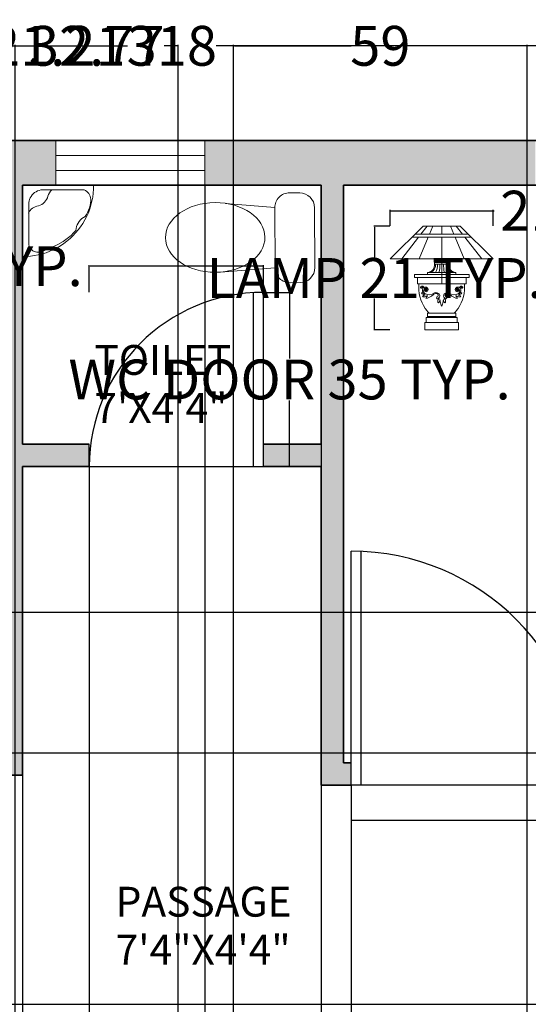
# Model space of a CAD drawing. Units: inches. Extents: x -24 to 368, y -370 to 58.
# Tile 8 of 9: x 133 to 235, y -140 to 58. Entities that reach past the tile are written whole.
import ezdxf

# ---------------------------------------------------------------- set-up
doc = ezdxf.new("R2010")
doc.units = ezdxf.units.IN
doc.header["$MEASUREMENT"] = 0
for name, color, linetype, lineweight in [('A-ANNO-DIMS', 2, 'Continuous', 18), ('A-AREA-IDEN', 7, 'Continuous', 18), ('A-FLOR-FIXT', 8, 'Continuous', 18), ('A-WALL', 7, 'Continuous', 35), ('Furniture', 7, 'Continuous', 15)]:
    doc.layers.add(name, color=color, linetype=linetype, lineweight=lineweight)
for name, color, linetype, lineweight, true_color in [('A-DOOR', 40, 'Continuous', 25, 0xf8d731), ('A-GLAZ', 30, 'Continuous', 18, 0xf26722), ('A-WALL-PATT', 18, 'Continuous', 13, 0x000000)]:
    doc.layers.add(name, color=color, linetype=linetype, lineweight=lineweight, true_color=true_color)
doc.styles.get("Standard").update_dxf_attribs({"font": 'arial.ttf'})
doc.dimstyles.get("Standard").update_dxf_attribs({"dimtxt": 8, "dimasz": 0.18, "dimexe": 0.18, "dimexo": 0.0625, "dimgap": 0.09, "dimtad": 0, "dimtih": 1, "dimtoh": 1, "dimdec": 4, "dimzin": 0, "dimdsep": 46, "dimlunit": 3, "dimtxsty": 'Standard', "dimcen": 0.09, "dimclre": 5, "dimclrt": 6, "dimadec": 0, "dimazin": 0, "dimtfac": 1, "dimtdec": 4, "dimtofl": 0, "dimtmove": 0, "dimatfit": 3, "dimfxl": 1, "dimtolj": 1, "dimtzin": 0, "dimarcsym": 0})

# ---------------------------------------------------------------- blocks, each defined once
blk = doc.blocks.new('LAMP-BEDSIDE')
for p, q in [((6.65, 20.8), (0, 14.26)), ((6.17, 19.19), (7.42, 20.8)), ((6.65, 20.8), (14.09, 20.8)), ((8.59, 20.8), (7.91, 19.19)), ((10.37, 20.8), (10.37, 19.19)), ((12.15, 20.8), (12.83, 19.19)), ((14.57, 19.19), (13.31, 20.8)), ((14.09, 20.8), (20.74, 14.26)), ((2.33, 14.26), (5.71, 18.6)), ((4.42, 18.6), (16.32, 18.6)), ((5.01, 19.19), (15.72, 19.19)), ((7.66, 18.6), (5.82, 14.26)), ((10.37, 18.6), (10.37, 9.21)), ((13.08, 18.6), (14.92, 14.26)), ((18.41, 14.26), (15.02, 18.6)), ((0, 14.26), (20.74, 14.26)), ((9.6, 14.09), (11.14, 14.09)), ((9.6, 14.09), (9.6, 13.52)), ((11.14, 14.09), (11.14, 13.52)), ((8.92, 13.52), (11.81, 13.52)), ((8.92, 13.52), (8.92, 13.19)), ((8.92, 13.19), (11.81, 13.19)), ((11.81, 13.52), (11.81, 13.19)), ((4.88, 11.13), (4.88, 10.49)), ((4.88, 11.13), (15.86, 11.13)), ((4.88, 10.49), (15.86, 10.49)), ((5.48, 10.49), (5.48, 9.21)), ((7.53, 11.52), (13.2, 11.52)), ((7.53, 11.52), (7.53, 11.13)), ((13.2, 11.52), (13.2, 11.13)), ((15.26, 10.49), (15.26, 9.21)), ((15.86, 11.13), (15.86, 10.49)), ((5.48, 9.21), (15.26, 9.21)), ((5.76, 9.21), (5.76, 8.59)), ((14.98, 9.21), (14.98, 8.59)), ((7.24, 2.43), (10.37, 2.43)), ((7.24, 2.43), (7.24, 1.48)), ((7.53, 3.34), (10.37, 3.34)), ((7.53, 3.34), (7.53, 2.65)), ((7.53, 2.65), (10.37, 2.65)), ((13.2, 3.34), (10.37, 3.34)), ((13.2, 2.65), (10.37, 2.65)), ((13.5, 2.43), (10.37, 2.43)), ((13.2, 3.34), (13.2, 2.65)), ((13.5, 2.43), (13.5, 1.48)), ((6.96, 1.48), (6.96, 0)), ((6.96, 1.48), (7.24, 1.48)), ((6.96, 0), (10.37, 0)), ((7.24, 1.48), (10.37, 1.48)), ((13.5, 1.48), (10.37, 1.48)), ((13.77, 0), (10.37, 0)), ((13.77, 1.48), (13.5, 1.48)), ((13.77, 1.48), (13.77, 0))]:
    blk.add_line(p, q)
for centre, radius, start, end in [((7.4, 13.04), 1.53, 274.9221, 5.4044), ((7.51, 13), 1.63, 295.0919, 6.6681), ((6.74, 12.97), 2.77, 328.5732, 4.5839), ((4.28, 12.92), 5.72, 345.8511, 2.7031), ((16.46, 12.92), 5.72, 177.2969, 194.1489), ((14, 12.97), 2.77, 175.4161, 211.4268), ((13.22, 13), 1.63, 173.3319, 244.9081), ((13.33, 13.04), 1.53, 174.5956, 265.0779), ((13.2, 8.5), 7.44, 179.3119, 219.4824), ((6.29, 8.51), 0.158, 124.9924, 335.335), ((6.45, 8.39), 0.355, 11.1092, 135.0155), ((6.39, 8.42), 0.0502, 145.048, 23.2806), ((6.51, 8.39), 0.171, 352.7452, 159.4145), ((7.39, 7.88), 0.87, 145.6908, 234.6789), ((7.4, 7.83), 0.668, 137.9008, 234.3868), ((7.12, 8.07), 0.5, 320.8911, 130.3323), ((7.11, 7.94), 0.236, 29.1955, 234.854), ((7.14, 8.08), 0.309, 326.7711, 139.3622), ((7.2, 8), 0.128, 26.7504, 223.4128), ((13.61, 8.07), 0.5, 49.6677, 219.1089), ((7.54, 8.5), 7.44, 320.5176, 0.6881), ((13.6, 8.08), 0.309, 40.6378, 213.2289), ((13.63, 7.94), 0.236, 305.146, 150.8045), ((13.54, 8), 0.128, 316.5872, 153.2496), ((13.34, 7.83), 0.668, 305.6132, 42.0992), ((13.34, 7.88), 0.87, 305.3211, 34.3092), ((14.29, 8.39), 0.355, 44.9845, 168.8908), ((14.23, 8.39), 0.171, 20.5855, 187.2548), ((14.45, 8.51), 0.158, 204.665, 55.0076), ((14.35, 8.42), 0.0502, 156.7194, 34.952), ((6.44, 6.9), 0.527, 30.7639, 106.5031), ((6.66, 7.53), 0.391, 199.4301, 258.0626), ((6.99, 6.45), 0.534, 81.7725, 150.3347), ((6.86, 7.15), 0.552, 231.7834, 300.6647), ((6.55, 6.3), 0.85, 53.0509, 88.4488), ((7.24, 8), 0.363, 223.4201, 318.9658), ((7.88, 8.48), 1.48, 232.7522, 313.7075), ((7.25, 8.05), 0.203, 224.103, 315.897), ((7.49, 6.32), 0.495, 75.8737, 133.8842), ((7.68, 6.3), 0.502, 98.3136, 177.606), ((7.04, 8.37), 2.05, 274.0547, 309.0162), ((5.53, 10.82), 4.92, 304.6293, 311.2979), ((9.22, 6.66), 0.644, 58.6818, 132.9572), ((9.12, 6.87), 0.587, 71.5671, 111.734), ((9.36, 6.81), 0.621, 342.0461, 94.8157), ((9.69, 6.38), 0.339, 108.5318, 204.8769), ((9.33, 6.92), 0.689, 273.9841, 333.6418), ((9.32, 6.94), 0.352, 316.7375, 49.0095), ((10.14, 5.79), 0.564, 138.2432, 224.6957), ((9.31, 6.66), 0.643, 310.3655, 356.3809), ((8.93, 6.11), 1.09, 318.697, 356.3018), ((9.3, 5.7), 0.788, 353.0671, 25.9825), ((11.43, 5.7), 0.788, 154.0175, 186.9329), ((11.81, 6.11), 1.09, 183.6982, 221.303), ((11.38, 6.81), 0.621, 85.1843, 197.9539), ((11.41, 6.92), 0.689, 206.3582, 266.0159), ((11.43, 6.66), 0.643, 183.6191, 229.6345), ((10.59, 5.79), 0.564, 315.3043, 41.7568), ((11.41, 6.94), 0.352, 130.9905, 223.2625), ((11.05, 6.38), 0.339, 335.1231, 71.4682), ((11.52, 6.66), 0.644, 47.0428, 121.3182), ((11.62, 6.87), 0.587, 68.266, 108.4329), ((12.85, 8.48), 1.48, 226.2925, 307.2478), ((15.2, 10.82), 4.92, 228.7021, 235.3707), ((13.7, 8.37), 2.05, 230.9838, 265.9453), ((13.25, 6.32), 0.495, 46.1158, 104.1263), ((13.05, 6.3), 0.502, 2.394, 81.6864), ((13.5, 8), 0.363, 221.0342, 316.5799), ((13.48, 8.05), 0.203, 224.103, 315.897), ((13.87, 7.15), 0.552, 239.3353, 308.2166), ((14.18, 6.3), 0.85, 91.5512, 126.9491), ((13.75, 6.45), 0.534, 29.6653, 98.2275), ((14.3, 6.9), 0.527, 73.4969, 149.2361), ((14.08, 7.53), 0.391, 281.9374, 340.5699), ((12.16, 5.83), 2.09, 186.3334, 210.8958), ((8.58, 5.83), 2.09, 329.1042, 353.6666), ((7.29, 2.67), 0.245, 257.4164, 350.592), ((10.43, 6.05), 3.74, 217.4462, 226.2556), ((10.31, 6.05), 3.74, 313.7444, 322.5538), ((10.31, 6.05), 3.74, 313.7444, 322.5538), ((13.45, 2.67), 0.245, 189.408, 282.5836)]:
    blk.add_arc(centre, radius, start, end)
blk = doc.blocks.new('WINDOW-30')
for p, q in [((0, 9), (30, 9)), ((0, 0), (0, 9)), ((30, 9), (30, 0)), ((0, 6), (30, 6)), ((0, 3), (30, 3)), ((30, 0), (0, 0))]:
    blk.add_line(p, q)
blk = doc.blocks.new('DOOR-SINGLE-35')
for p, q in [((0, 35), (0, 0)), ((0, 35), (4.5, 35)), ((0, 2), (35, 2)), ((0, 0), (35, 0)), ((0, 0), (4.5, 0))]:
    blk.add_line(p, q)
blk.add_arc((0, 0), 35, 0, 90)
blk = doc.blocks.new('DOOR-SINGLE-47')
for p, q in [((0, 0), (0, 47)), ((2, 0), (2, 47)), ((47, 0), (0, 0))]:
    blk.add_line(p, q)
blk.add_arc((0, 0), 47, 0, 90)
blk = doc.blocks.new('*D13')
at = {"layer": 'A-ANNO-DIMS', "color": 5, "lineweight": -2, "transparency": 16777216}
for p, q in [((206.97, 16.43), (203.73, 16.43)), ((206.97, -4.37), (203.73, -4.37))]:
    blk.add_line(p, q, dxfattribs=at)
at = {"layer": 'A-ANNO-DIMS', "color": 0, "lineweight": -2, "transparency": 16777216}
for p, q in [((203.91, 16.25), (203.91, 10.14)), ((203.91, -4.19), (203.91, 1.92))]:
    blk.add_line(p, q, dxfattribs=at)
at = {"layer": 'A-ANNO-DIMS', "color": 0, "transparency": 16777216}
for points in [[(203.88, 16.25), (203.94, 16.25), (203.91, 16.43)], [(203.88, -4.19), (203.94, -4.19), (203.91, -4.37)]]:
    blk.add_solid(points, dxfattribs=at)
at = {"layer": 'Defpoints', "color": 0, "transparency": 16777216}
for p in [(203.91, 16.43), (207.03, 16.43), (207.03, -4.37)]:
    blk.add_point(p, dxfattribs=at)
at = {"layer": 'A-ANNO-DIMS', "color": 6, "transparency": 16777216, "insert": (203.91, 6.03), "char_height": 8, "attachment_point": 5}
blk.add_mtext('\\A1;LAMP 21 TYP.', dxfattribs=at)
blk = doc.blocks.new('*D14')
at = {"layer": 'A-ANNO-DIMS', "color": 5, "lineweight": -2, "transparency": 16777216}
for p, q in [((207.03, 16.49), (207.03, 19.73)), ((227.77, 16.49), (227.77, 19.73))]:
    blk.add_line(p, q, dxfattribs=at)
at = {"layer": 'A-ANNO-DIMS', "color": 0, "lineweight": -2, "transparency": 16777216}
for p, q in [((207.21, 19.55), (227.59, 19.55)), ((227.77, 19.55), (227.95, 19.55))]:
    blk.add_line(p, q, dxfattribs=at)
at = {"layer": 'A-ANNO-DIMS', "color": 0, "transparency": 16777216}
for points in [[(207.21, 19.58), (207.21, 19.52), (207.03, 19.55)], [(227.59, 19.58), (227.59, 19.52), (227.77, 19.55)]]:
    blk.add_solid(points, dxfattribs=at)
at = {"layer": 'Defpoints', "color": 0, "transparency": 16777216}
for p in [(227.77, 19.55), (207.03, 16.43), (227.77, 16.43)]:
    blk.add_point(p, dxfattribs=at)
at = {"layer": 'A-ANNO-DIMS', "color": 6, "transparency": 16777216, "insert": (247.58, 19.55), "char_height": 8, "attachment_point": 5}
blk.add_mtext('\\A1;21 TYP.', dxfattribs=at)
blk = doc.blocks.new('*D19')
at = {"layer": 'A-ANNO-DIMS', "color": 5, "lineweight": -2, "transparency": 16777216}
for p, q in [((199.21, -95.92), (199.21, -103.09)), ((246.21, -95.92), (246.21, -103.09))]:
    blk.add_line(p, q, dxfattribs=at)
at = {"layer": 'A-ANNO-DIMS', "color": 0, "lineweight": -2, "transparency": 16777216}
for p, q in [((199.39, -102.91), (246.03, -102.91)), ((246.21, -102.91), (246.39, -102.91))]:
    blk.add_line(p, q, dxfattribs=at)
at = {"layer": 'A-ANNO-DIMS', "color": 0, "transparency": 16777216}
for points in [[(199.39, -102.88), (199.39, -102.94), (199.21, -102.91)], [(246.03, -102.88), (246.03, -102.94), (246.21, -102.91)]]:
    blk.add_solid(points, dxfattribs=at)
at = {"layer": 'Defpoints', "color": 0, "transparency": 16777216}
for p in [(199.21, -95.86), (246.21, -95.86), (246.21, -102.91)]:
    blk.add_point(p, dxfattribs=at)
at = {"layer": 'A-ANNO-DIMS', "color": 6, "transparency": 16777216, "insert": (306.3, -102.91), "char_height": 8, "attachment_point": 5}
blk.add_mtext('\\A1;SINGLE DOOR 47 TYP.', dxfattribs=at)
blk = doc.blocks.new('*D23')
at = {"layer": 'A-ANNO-DIMS', "color": 5, "lineweight": -2, "transparency": 16777216}
for p, q in [((181.63, 3.14), (187, 3.14)), ((181.63, -31.86), (187, -31.86))]:
    blk.add_line(p, q, dxfattribs=at)
at = {"layer": 'A-ANNO-DIMS', "color": 0, "lineweight": -2, "transparency": 16777216}
for p, q in [((186.82, 2.96), (186.82, -10.13)), ((186.82, -31.68), (186.82, -18.59))]:
    blk.add_line(p, q, dxfattribs=at)
at = {"layer": 'A-ANNO-DIMS', "color": 0, "transparency": 16777216}
for points in [[(186.79, 2.96), (186.85, 2.96), (186.82, 3.14)], [(186.79, -31.68), (186.85, -31.68), (186.82, -31.86)]]:
    blk.add_solid(points, dxfattribs=at)
at = {"layer": 'Defpoints', "color": 0, "transparency": 16777216}
for p in [(181.57, 3.14), (186.82, 3.14), (181.57, -31.86)]:
    blk.add_point(p, dxfattribs=at)
at = {"layer": 'A-ANNO-DIMS', "color": 6, "transparency": 16777216, "insert": (186.82, -14.36), "char_height": 8, "attachment_point": 5}
blk.add_mtext('\\A1;WC DOOR 35 TYP.', dxfattribs=at)
blk = doc.blocks.new('*D24')
at = {"layer": 'A-ANNO-DIMS', "color": 0, "lineweight": -2, "transparency": 16777216}
for p, q in [((146.57, 8.39), (146.39, 8.39)), ((181.39, 8.39), (146.75, 8.39))]:
    blk.add_line(p, q, dxfattribs=at)
at = {"layer": 'A-ANNO-DIMS', "color": 5, "lineweight": -2, "transparency": 16777216}
for p, q in [((146.57, 3.21), (146.57, 8.57)), ((181.57, 3.21), (181.57, 8.57))]:
    blk.add_line(p, q, dxfattribs=at)
at = {"layer": 'A-ANNO-DIMS', "color": 0, "transparency": 16777216}
for points in [[(146.75, 8.42), (146.75, 8.36), (146.57, 8.39)], [(181.39, 8.42), (181.39, 8.36), (181.57, 8.39)]]:
    blk.add_solid(points, dxfattribs=at)
at = {"layer": 'Defpoints', "color": 0, "transparency": 16777216}
for p in [(146.57, 8.39), (146.57, 3.14), (181.57, 3.14)]:
    blk.add_point(p, dxfattribs=at)
at = {"layer": 'A-ANNO-DIMS', "color": 6, "transparency": 16777216, "insert": (126.83, 8.39), "char_height": 8, "attachment_point": 5}
blk.add_mtext('\\A1;35 TYP.', dxfattribs=at)
blk = doc.blocks.new('*D25')
at = {"layer": 'A-ANNO-DIMS', "color": 5, "lineweight": -2, "transparency": 16777216}
for p, q in [((4.16, 33.71), (4.16, 52.85)), ((322.16, 33.71), (322.16, 52.85))]:
    blk.add_line(p, q, dxfattribs=at)
at = {"layer": 'A-ANNO-DIMS', "color": 0, "lineweight": -2, "transparency": 16777216}
for p, q in [((4.34, 52.67), (154.23, 52.67)), ((321.98, 52.67), (172.1, 52.67))]:
    blk.add_line(p, q, dxfattribs=at)
at = {"layer": 'A-ANNO-DIMS', "color": 0, "transparency": 16777216}
for points in [[(4.34, 52.7), (4.34, 52.64), (4.16, 52.67)], [(321.98, 52.7), (321.98, 52.64), (322.16, 52.67)]]:
    blk.add_solid(points, dxfattribs=at)
at = {"layer": 'Defpoints', "color": 0, "transparency": 16777216}
for p in [(322.16, 52.67), (4.16, 33.64), (322.16, 33.64)]:
    blk.add_point(p, dxfattribs=at)
at = {"layer": 'A-ANNO-DIMS', "color": 6, "transparency": 16777216, "insert": (163.16, 52.67), "char_height": 8, "attachment_point": 5}
blk.add_mtext('\\A1;318', dxfattribs=at)
blk = doc.blocks.new('*D42')
at = {"layer": 'A-ANNO-DIMS', "color": 5, "lineweight": -2, "transparency": 16777216}
for p, q in [((169.81, 24.59), (169.81, -363.55)), ((193.16, 24.58), (193.16, -363.55))]:
    blk.add_line(p, q, dxfattribs=at)
at = {"layer": 'A-ANNO-DIMS', "color": 0, "lineweight": -2, "transparency": 16777216}
for p, q in [((169.99, -363.37), (192.98, -363.37)), ((193.16, -363.37), (193.34, -363.37))]:
    blk.add_line(p, q, dxfattribs=at)
at = {"layer": 'A-ANNO-DIMS', "color": 0, "transparency": 16777216}
for points in [[(169.99, -363.34), (169.99, -363.4), (169.81, -363.37)], [(192.98, -363.34), (192.98, -363.4), (193.16, -363.37)]]:
    blk.add_solid(points, dxfattribs=at)
at = {"layer": 'Defpoints', "color": 0, "transparency": 16777216}
for p in [(169.81, 24.65), (193.16, 24.64), (193.16, -363.37)]:
    blk.add_point(p, dxfattribs=at)
at = {"layer": 'A-ANNO-DIMS', "color": 6, "transparency": 16777216, "insert": (207.03, -363.37), "char_height": 8, "attachment_point": 5}
blk.add_mtext('\\A1;23.35', dxfattribs=at)
blk = doc.blocks.new('*D44')
at = {"layer": 'A-ANNO-DIMS', "color": 5, "lineweight": -2, "transparency": 16777216}
for p, q in [((13.22, -61.1), (341.36, -61.1)), ((13.22, -89.36), (341.36, -89.36))]:
    blk.add_line(p, q, dxfattribs=at)
at = {"layer": 'A-ANNO-DIMS', "color": 0, "lineweight": -2, "transparency": 16777216}
for p, q in [((341.18, -61.28), (341.18, -71.05)), ((341.18, -89.18), (341.18, -79.4))]:
    blk.add_line(p, q, dxfattribs=at)
at = {"layer": 'A-ANNO-DIMS', "color": 0, "transparency": 16777216}
for points in [[(341.15, -61.28), (341.21, -61.28), (341.18, -61.1)], [(341.15, -89.18), (341.21, -89.18), (341.18, -89.36)]]:
    blk.add_solid(points, dxfattribs=at)
at = {"layer": 'Defpoints', "color": 0, "transparency": 16777216}
for p in [(13.16, -61.1), (341.18, -61.1), (13.16, -89.36)]:
    blk.add_point(p, dxfattribs=at)
at = {"layer": 'A-ANNO-DIMS', "color": 6, "transparency": 16777216, "insert": (341.18, -75.23), "char_height": 8, "attachment_point": 5}
blk.add_mtext('\\A1;28.26', dxfattribs=at)
blk = doc.blocks.new('*D51')
at = {"layer": 'A-ANNO-DIMS', "color": 5, "lineweight": -2, "transparency": 16777216}
for p, q in [((175.57, -303.29), (175.57, 52.85)), ((234.57, -303.29), (234.57, 52.85))]:
    blk.add_line(p, q, dxfattribs=at)
at = {"layer": 'A-ANNO-DIMS', "color": 0, "lineweight": -2, "transparency": 16777216}
for p, q in [((175.75, 52.67), (199.24, 52.67)), ((234.39, 52.67), (210.9, 52.67))]:
    blk.add_line(p, q, dxfattribs=at)
at = {"layer": 'A-ANNO-DIMS', "color": 0, "transparency": 16777216}
for points in [[(175.75, 52.7), (175.75, 52.64), (175.57, 52.67)], [(234.39, 52.7), (234.39, 52.64), (234.57, 52.67)]]:
    blk.add_solid(points, dxfattribs=at)
at = {"layer": 'Defpoints', "color": 0, "transparency": 16777216}
for p in [(234.57, 52.67), (175.57, -303.36), (234.57, -303.36)]:
    blk.add_point(p, dxfattribs=at)
at = {"layer": 'A-ANNO-DIMS', "color": 6, "transparency": 16777216, "insert": (205.07, 52.67), "char_height": 8, "attachment_point": 5}
blk.add_mtext('\\A1;59', dxfattribs=at)
blk = doc.blocks.new('*D55')
at = {"layer": 'A-ANNO-DIMS', "color": 5, "lineweight": -2, "transparency": 16777216}
for p, q in [((131.66, -152.29), (131.66, 52.85)), ((164.43, -152.29), (164.43, 52.85))]:
    blk.add_line(p, q, dxfattribs=at)
at = {"layer": 'A-ANNO-DIMS', "color": 0, "lineweight": -2, "transparency": 16777216}
for p, q in [((131.84, 52.67), (134.46, 52.67)), ((164.25, 52.67), (161.63, 52.67))]:
    blk.add_line(p, q, dxfattribs=at)
at = {"layer": 'A-ANNO-DIMS', "color": 0, "transparency": 16777216}
for points in [[(131.84, 52.7), (131.84, 52.64), (131.66, 52.67)], [(164.25, 52.7), (164.25, 52.64), (164.43, 52.67)]]:
    blk.add_solid(points, dxfattribs=at)
at = {"layer": 'Defpoints', "color": 0, "transparency": 16777216}
for p in [(164.43, 52.67), (131.66, -152.36), (164.43, -152.36)]:
    blk.add_point(p, dxfattribs=at)
at = {"layer": 'A-ANNO-DIMS', "color": 6, "transparency": 16777216, "insert": (148.05, 52.67), "char_height": 8, "attachment_point": 5}
blk.add_mtext('\\A1;32.77', dxfattribs=at)
blk = doc.blocks.new('*D58')
at = {"layer": 'A-ANNO-DIMS', "color": 5, "lineweight": -2, "transparency": 16777216}
for p, q in [((133.16, -31.92), (133.16, -363.55)), ((146.57, -31.92), (146.57, -363.55))]:
    blk.add_line(p, q, dxfattribs=at)
at = {"layer": 'A-ANNO-DIMS', "color": 0, "lineweight": -2, "transparency": 16777216}
for p, q in [((133.34, -363.37), (146.39, -363.37)), ((146.57, -363.37), (146.75, -363.37))]:
    blk.add_line(p, q, dxfattribs=at)
at = {"layer": 'A-ANNO-DIMS', "color": 0, "transparency": 16777216}
for points in [[(133.34, -363.34), (133.34, -363.4), (133.16, -363.37)], [(146.39, -363.34), (146.39, -363.4), (146.57, -363.37)]]:
    blk.add_solid(points, dxfattribs=at)
at = {"layer": 'Defpoints', "color": 0, "transparency": 16777216}
for p in [(133.16, -31.86), (146.57, -31.86), (146.57, -363.37)]:
    blk.add_point(p, dxfattribs=at)
at = {"layer": 'A-ANNO-DIMS', "color": 6, "transparency": 16777216, "insert": (163.1, -363.37), "char_height": 8, "attachment_point": 5}
blk.add_mtext('\\A1;13.405', dxfattribs=at)
blk = doc.blocks.new('*D59')
at = {"layer": 'A-ANNO-DIMS', "color": 5, "lineweight": -2, "transparency": 16777216}
for p, q in [((246.6, -139.91), (-15.03, -139.91)), ((246.6, -147.86), (-15.03, -147.86))]:
    blk.add_line(p, q, dxfattribs=at)
at = {"layer": 'A-ANNO-DIMS', "color": 0, "lineweight": -2, "transparency": 16777216}
for p, q in [((-14.85, -139.91), (-14.85, -139.73)), ((-14.85, -139.73), (-14.67, -139.73)), ((-14.85, -147.68), (-14.85, -140.09))]:
    blk.add_line(p, q, dxfattribs=at)
at = {"layer": 'A-ANNO-DIMS', "color": 0, "transparency": 16777216}
for points in [[(-14.88, -140.09), (-14.82, -140.09), (-14.85, -139.91)], [(-14.88, -147.68), (-14.82, -147.68), (-14.85, -147.86)]]:
    blk.add_solid(points, dxfattribs=at)
at = {"layer": 'Defpoints', "color": 0, "transparency": 16777216}
for p in [(-14.85, -139.91), (246.66, -139.91), (246.66, -147.86)]:
    blk.add_point(p, dxfattribs=at)
at = {"layer": 'A-ANNO-DIMS', "color": 6, "transparency": 16777216, "insert": (-4.2, -139.73), "char_height": 8, "attachment_point": 5}
blk.add_mtext('\\A1;7.95', dxfattribs=at)
blk = doc.blocks.new('*D60')
at = {"layer": 'A-ANNO-DIMS', "color": 5, "lineweight": -2, "transparency": 16777216}
for p, q in [((133.16, -93.92), (133.16, -363.55)), ((193.16, -95.92), (193.16, -363.55))]:
    blk.add_line(p, q, dxfattribs=at)
at = {"layer": 'A-ANNO-DIMS', "color": 0, "lineweight": -2, "transparency": 16777216}
for p, q in [((133.34, -363.37), (157.33, -363.37)), ((192.98, -363.37), (168.99, -363.37))]:
    blk.add_line(p, q, dxfattribs=at)
at = {"layer": 'A-ANNO-DIMS', "color": 0, "transparency": 16777216}
for points in [[(133.34, -363.34), (133.34, -363.4), (133.16, -363.37)], [(192.98, -363.34), (192.98, -363.4), (193.16, -363.37)]]:
    blk.add_solid(points, dxfattribs=at)
at = {"layer": 'Defpoints', "color": 0, "transparency": 16777216}
for p in [(133.16, -93.86), (193.16, -95.86), (193.16, -363.37)]:
    blk.add_point(p, dxfattribs=at)
at = {"layer": 'A-ANNO-DIMS', "color": 6, "transparency": 16777216, "insert": (163.16, -363.37), "char_height": 8, "attachment_point": 5}
blk.add_mtext('\\A1;60', dxfattribs=at)
blk = doc.blocks.new('*D65')
at = {"layer": 'A-ANNO-DIMS', "color": 5, "lineweight": -2, "transparency": 16777216}
for p, q in [((105.95, -335.29), (105.95, 52.85)), ((127.16, -335.29), (127.16, 52.85))]:
    blk.add_line(p, q, dxfattribs=at)
at = {"layer": 'A-ANNO-DIMS', "color": 0, "lineweight": -2, "transparency": 16777216}
for p, q in [((106.13, 52.67), (126.98, 52.67)), ((127.16, 52.67), (127.34, 52.67))]:
    blk.add_line(p, q, dxfattribs=at)
at = {"layer": 'A-ANNO-DIMS', "color": 0, "transparency": 16777216}
for points in [[(106.13, 52.7), (106.13, 52.64), (105.95, 52.67)], [(126.98, 52.7), (126.98, 52.64), (127.16, 52.67)]]:
    blk.add_solid(points, dxfattribs=at)
at = {"layer": 'Defpoints', "color": 0, "transparency": 16777216}
for p in [(127.16, 52.67), (105.95, -335.36), (127.16, -335.36)]:
    blk.add_point(p, dxfattribs=at)
at = {"layer": 'A-ANNO-DIMS', "color": 6, "transparency": 16777216, "insert": (140.23, 52.67), "char_height": 8, "attachment_point": 5}
blk.add_mtext('\\A1;21.21', dxfattribs=at)
blk = doc.blocks.new('*D70')
at = {"layer": 'A-ANNO-DIMS', "color": 5, "lineweight": -2, "transparency": 16777216}
for p, q in [((193.16, -95.92), (193.16, -363.55)), ((199.21, -95.92), (199.21, -363.55))]:
    blk.add_line(p, q, dxfattribs=at)
at = {"layer": 'A-ANNO-DIMS', "color": 0, "lineweight": -2, "transparency": 16777216}
for p, q in [((193.34, -363.37), (199.03, -363.37)), ((199.21, -363.37), (199.39, -363.37))]:
    blk.add_line(p, q, dxfattribs=at)
at = {"layer": 'A-ANNO-DIMS', "color": 0, "transparency": 16777216}
for points in [[(193.34, -363.34), (193.34, -363.4), (193.16, -363.37)], [(199.03, -363.34), (199.03, -363.4), (199.21, -363.37)]]:
    blk.add_solid(points, dxfattribs=at)
at = {"layer": 'Defpoints', "color": 0, "transparency": 16777216}
for p in [(193.16, -95.86), (199.21, -95.86), (199.21, -363.37)]:
    blk.add_point(p, dxfattribs=at)
at = {"layer": 'A-ANNO-DIMS', "color": 6, "transparency": 16777216, "insert": (212.23, -363.37), "char_height": 8, "attachment_point": 5}
blk.add_mtext('\\A1;6.051', dxfattribs=at)

msp = doc.modelspace()

# ---------------------------------------------------------------- hatches: boundary and pattern name
at = {"layer": 'A-WALL-PATT'}
h = msp.add_hatch(color=256, dxfattribs=at)
h.dxf.hatch_style = 1
h.paths.add_polyline_path([(13.1621, -93.8573), (80.4499, -93.8573), (80.4499, -89.3573), (13.1621, -89.3573), (13.1621, -61.0987), (4.1621, -61.0987), (4.1621, -149.8573), (13.1621, -149.8573)])
h.paths.add_polyline_path([(146.5668, -27.3573), (133.1621, -27.3573), (133.1621, 10.3323), (133.1272, 10.3313), (133.1621, 24.6427), (139.8141, 24.6427), (139.8141, 33.6427), (95.3329, 33.6427), (95.3329, 24.6427), (128.6621, 24.6427), (128.6621, -89.3573), (127.4499, -89.3573), (127.4499, -93.8573), (133.1621, -93.8573), (133.1621, -31.8573), (146.5668, -31.8573)])
h.paths.add_polyline_path([(197.6621, 24.6427), (236.2134, 24.6427), (236.2134, 33.6427), (169.8141, 33.6427), (169.8141, 24.6427), (193.1621, 24.6427), (193.1621, -27.3573), (181.5668, -27.3573), (181.5668, -31.8573), (193.1621, -31.8573), (193.1621, -95.8573), (199.2127, -95.8573), (199.2127, -91.3573), (197.6621, -91.3573)])
h.paths.add_polyline_path([(322.1621, -52.531), (313.1621, -52.531), (313.1621, -91.3573), (246.2127, -91.3573), (246.2127, -95.8573), (246.6621, -95.8573), (246.6621, -104.9077), (251.1621, -104.9077), (251.1621, -95.8573), (313.1621, -95.8573), (313.1621, -105.6922), (317.6621, -105.6922), (322.1621, -105.6922)])
h.paths.add_polyline_path([(322.1621, -135.6922), (313.1621, -135.6922), (313.1621, -147.8573), (251.1621, -147.8573), (251.1621, -139.9077), (246.6621, -139.9077), (246.6621, -147.8573), (199.43, -147.8573), (199.43, -152.3573), (313.1621, -152.3573), (313.1621, -194.6142), (317.6621, -194.6142), (322.1621, -194.6142)])
h.paths.add_polyline_path([(322.1621, -241.6142), (313.1621, -241.6142), (313.1621, -275.3573), (287.3912, -275.3573), (287.3912, -279.8573), (313.1621, -279.8573), (313.1621, -335.3573), (298.077, -335.3573), (298.077, -344.3573), (322.1621, -344.3573)])
h.paths.add_polyline_path([(263.077, -335.3573), (241.1621, -335.3573), (241.1621, -279.8573), (252.3912, -279.8573), (252.3912, -275.3573), (236.6621, -275.3573), (236.6621, -298.8573), (234.5689, -298.8573), (234.5689, -303.3573), (236.6621, -303.3573), (236.6621, -344.3573), (263.077, -344.3573), (263.077, -339.8573)])
h.paths.add_polyline_path([(175.5689, -298.8573), (131.6621, -298.8573), (131.6621, -152.3573), (164.43, -152.3573), (164.43, -147.8573), (127.1621, -147.8573), (127.1621, -232.8573), (117.1621, -232.8573), (117.1621, -237.3573), (127.1621, -237.3573), (127.1621, -335.3573), (84.4055, -335.3573), (84.4055, -344.3573), (131.6621, -344.3573), (131.6621, -303.3573), (175.5689, -303.3573)])
h.paths.add_polyline_path([(70.1621, -232.8573), (13.1621, -232.8573), (13.1621, -196.8573), (4.1621, -196.8573), (4.1621, -257.9061), (13.1621, -257.9061), (13.1621, -237.3573), (70.1621, -237.3573)])
h.paths.add_polyline_path([(13.1621, -304.9061), (4.1621, -304.9061), (4.1621, -344.3573), (37.4055, -344.3573), (37.4055, -335.3573), (13.1621, -335.3573)])
h.paths.add_polyline_path([(322.1621, 33.6427), (283.2134, 33.6427), (283.2134, 24.6427), (313.1621, 24.6427), (313.1621, 11.9273), (313.4656, 11.629), (313.1621, 11.629), (313.1621, -5.531), (322.1621, -5.531)])
h.paths.add_polyline_path([(48.3329, 33.6427), (4.1621, 33.6427), (4.1621, -14.0987), (13.1621, -14.0987), (13.1621, 24.6427), (48.3329, 24.6427)])

# ---------------------------------------------------------------- linework, layer by layer
at = {"layer": 'A-DOOR'}
msp.add_line((199.2127, -95.8573), (199.2127, -91.3573), dxfattribs=at)
at = {"layer": 'A-FLOR-FIXT'}
for p, q in [((133.1272, 10.3313), (133.1621, 24.6427)), ((133.1621, 24.6427), (147.4386, 24.6427)), ((147.4269, 23.8392), (147.3571, 23.0357)), ((147.4269, 23.8392), (147.4386, 24.6427)), ((134.5711, 21.8247), (134.478, 21.4986)), ((134.7108, 22.1391), (134.5711, 21.8247)), ((134.8739, 22.4302), (134.7108, 22.1391)), ((135.0835, 22.7097), (134.8739, 22.4302)), ((135.3164, 22.9542), (135.0835, 22.7097)), ((135.5842, 23.1754), (135.3164, 22.9542)), ((135.8753, 23.3618), (135.5842, 23.1754)), ((136.1781, 23.5131), (135.8753, 23.3618)), ((136.5041, 23.6296), (136.1781, 23.5131)), ((136.5041, 23.6296), (136.8302, 23.7111)), ((136.8302, 23.7111), (137.0165, 23.7111)), ((137.0165, 23.7111), (145.5172, 23.7344)), ((137.9714, 21.8247), (137.7734, 21.5335)), ((138.1344, 22.1391), (137.9714, 21.8247)), ((138.2509, 22.4768), (138.1344, 22.1391)), ((138.379, 22.8261), (138.2509, 22.4768)), ((138.5536, 23.1638), (138.379, 22.8261)), ((138.7749, 23.4666), (138.5536, 23.1638)), ((139.0311, 23.7344), (138.7749, 23.4666)), ((145.785, 23.6063), (145.5172, 23.7344)), ((146.0412, 23.4316), (145.785, 23.6063)), ((146.2625, 23.222), (146.0412, 23.4316)), ((146.4604, 22.9891), (146.2625, 23.222)), ((146.6235, 22.7213), (146.4604, 22.9891)), ((146.7515, 22.4418), (146.6235, 22.7213)), ((146.8331, 22.1507), (146.7515, 22.4418)), ((146.868, 21.8479), (146.8331, 22.1507)), ((146.868, 21.5335), (146.868, 21.8479)), ((147.2523, 22.2322), (147.1009, 21.452)), ((147.3571, 23.0357), (147.2523, 22.2322)), ((186.8564, 23.1443), (188.8562, 23.1353)), ((134.4081, 21.1609), (134.3964, 20.8116)), ((134.3964, 13.2541), (134.3964, 20.8116)), ((134.478, 21.4986), (134.4081, 21.1609)), ((134.9088, 19.845), (134.6876, 19.6121)), ((135.1534, 20.0546), (134.9088, 19.845)), ((135.4212, 20.2177), (135.1534, 20.0546)), ((135.7123, 20.3458), (135.4212, 20.2177)), ((136.0151, 20.4273), (135.7123, 20.3458)), ((136.3644, 20.5088), (136.0151, 20.4273)), ((136.6905, 20.6485), (136.3644, 20.5088)), ((137.0049, 20.8116), (136.6905, 20.6485)), ((137.2843, 21.0212), (137.0049, 20.8116)), ((137.5522, 21.2541), (137.2843, 21.0212)), ((137.7734, 21.5335), (137.5522, 21.2541)), ((146.67, 19.9033), (146.3789, 19.1464)), ((146.5885, 20.1129), (146.4255, 19.6471)), ((146.7166, 20.5787), (146.5885, 20.1129)), ((146.9029, 20.6718), (146.67, 19.9033)), ((146.8098, 21.0561), (146.7166, 20.5787)), ((146.868, 21.5335), (146.8098, 21.0561)), ((147.1009, 21.452), (146.9029, 20.6718)), ((183.8429, 20.1579), (173.9706, 21.0205)), ((183.9019, 8.0604), (183.843, 20.1297)), ((191.8427, 20.15), (191.9016, 8.1086)), ((134.5012, 19.356), (134.3615, 19.0648)), ((134.6876, 19.6121), (134.5012, 19.356)), ((145.0631, 17.9586), (144.7719, 17.6908)), ((145.3775, 18.1798), (145.0631, 17.9586)), ((145.7268, 18.3778), (145.3775, 18.1798)), ((146.0529, 18.4127), (145.6919, 17.6908)), ((145.9946, 18.7854), (145.7268, 18.3778)), ((146.2275, 19.2046), (145.9946, 18.7854)), ((146.3789, 19.1464), (146.0529, 18.4127)), ((146.4255, 19.6471), (146.2275, 19.2046)), ((143.8986, 15.9673), (143.852, 15.5714)), ((143.9917, 16.3516), (143.8986, 15.9673)), ((144.1315, 16.7126), (143.9917, 16.3516)), ((144.3061, 17.0619), (144.1315, 16.7126)), ((144.5157, 17.388), (144.3061, 17.0619)), ((144.8302, 16.3283), (144.3527, 15.6879)), ((144.7719, 17.6908), (144.5157, 17.388)), ((145.2843, 17.0037), (144.8302, 16.3283)), ((145.6919, 17.6908), (145.2843, 17.0037)), ((142.408, 14.1507), (141.8607, 13.7432)), ((142.6992, 13.9411), (142.082, 13.4171)), ((142.9204, 14.5932), (142.408, 14.1507)), ((143.2814, 14.4884), (142.6992, 13.9411)), ((143.4095, 15.0707), (142.9204, 14.5932)), ((143.8287, 15.0707), (143.2814, 14.4884)), ((143.852, 15.5714), (143.4095, 15.0707)), ((144.3527, 15.6879), (143.8287, 15.0707)), ((134.3848, 12.963), (134.3964, 13.2541)), ((134.4197, 12.6719), (134.3848, 12.963)), ((134.5012, 12.3924), (134.4197, 12.6719)), ((134.6293, 12.1362), (134.5012, 12.3924)), ((134.7924, 11.8917), (134.6293, 12.1362)), ((134.9903, 11.6821), (134.7924, 11.8917)), ((139.1359, 12.241), (138.0296, 11.7403)), ((140.2305, 12.7767), (139.1359, 12.241)), ((140.0791, 12.0896), (139.3571, 11.717)), ((140.7661, 12.4855), (140.0791, 12.0896)), ((141.2901, 13.3822), (140.2305, 12.7767)), ((141.4415, 12.9397), (140.7661, 12.4855)), ((141.8607, 13.7432), (141.2901, 13.3822)), ((142.082, 13.4171), (141.4415, 12.9397)), ((133.9306, 10.3545), (133.1272, 10.3313)), ((134.7341, 10.4128), (133.9306, 10.3545)), ((135.526, 10.5176), (134.7341, 10.4128)), ((135.2232, 11.5074), (134.9903, 11.6821)), ((135.4794, 11.356), (135.2232, 11.5074)), ((135.7472, 11.2628), (135.4794, 11.356)), ((136.3178, 10.669), (135.526, 10.5176)), ((136.0384, 11.2046), (135.7472, 11.2628)), ((136.3295, 11.193), (136.0384, 11.2046)), ((137.098, 10.8669), (136.3178, 10.669)), ((136.6089, 11.2279), (136.3295, 11.193)), ((136.8884, 11.2978), (136.6089, 11.2279)), ((138.0296, 11.7403), (136.8884, 11.2978)), ((136.8884, 11.3094), (136.8884, 11.2978)), ((136.8884, 11.2978), (136.8884, 11.3094)), ((137.8666, 11.1115), (137.098, 10.8669)), ((138.6235, 11.3909), (137.8666, 11.1115)), ((139.3571, 11.717), (138.6235, 11.3909)), ((183.902, 8.0467), (172.9163, 7.2119)), ((188.93, 5.0941), (186.9302, 5.0752))]:
    msp.add_line(p, q, dxfattribs=at)
for centre, start, end in [((186.843, 20.1443), 89.743728, 180.279405), ((188.8428, 20.1354), 0.280253, 89.743728), ((186.9019, 8.0751), 180.279405, 270.540714), ((188.9017, 8.0939), 270.540714, 0.280253)]:
    msp.add_arc(centre, 3, start, end, dxfattribs=at)
msp.add_ellipse((171.8721, 14.1711), major_axis=(-9.9999, -0.0489), ratio=0.7, dxfattribs=at)
at = {"layer": 'A-WALL'}
for p, q in [((4.1621, 33.6427), (322.1621, 33.6427)), ((133.1621, 24.6427), (193.1621, 24.6427)), ((133.1621, -27.3573), (133.1621, 24.6427)), ((193.1621, 24.6427), (193.1621, -27.3573)), ((197.6621, 24.6427), (197.6621, -91.3573)), ((197.6621, 24.6427), (313.1621, 24.6427)), ((133.1621, -27.3573), (146.5668, -27.3573)), ((181.5668, -27.3573), (193.1621, -27.3573)), ((133.1621, -93.8573), (133.1621, -31.8573)), ((133.1621, -31.8573), (146.5668, -31.8573)), ((181.5668, -31.8573), (193.1621, -31.8573)), ((193.1621, -31.8573), (193.1621, -95.8573)), ((197.6621, -91.3573), (199.2127, -91.3573)), ((127.4499, -93.8573), (133.1621, -93.8573)), ((193.1621, -95.8573), (199.2127, -95.8573))]:
    msp.add_line(p, q, dxfattribs=at)

# ---------------------------------------------------------------- block references
at = {"layer": 'A-DOOR', "rotation": 90.00000000000006}
msp.add_blockref('DOOR-SINGLE-35', (181.5671, -31.8574), dxfattribs=at)
at = {"layer": 'A-DOOR'}
msp.add_blockref('DOOR-SINGLE-47', (199.213, -95.857), dxfattribs=at)
at = {"layer": 'A-GLAZ'}
msp.add_blockref('WINDOW-30', (139.814, 24.651), dxfattribs=at)
at = {"layer": 'Furniture'}
msp.add_blockref('LAMP-BEDSIDE', (207.0333, -4.3723), dxfattribs=at)

# ---------------------------------------------------------------- texts
at = {"layer": 'A-AREA-IDEN'}
for s, p in [('TOILET', (147.5907, -13.4367)), ('7\'X4\'4"', (147.5907, -23.0751)), ('PASSAGE', (151.8623, -122.2733)), ('7\'4"X4\'4"', (151.8623, -131.9118))]:
    msp.add_text(s, height=6, dxfattribs=at).set_placement(p)

# ---------------------------------------------------------------- dimensions: what is measured, and where the dimension line sits
at = {"layer": 'A-ANNO-DIMS'}
for base, p1, p2, override, picture, middle in [((322.1621, 52.6658), (4.1621, 33.6427), (322.1621, 33.6427), {"dimdec": 0, "dimlfac": 1, "dimrnd": 0, "dimzin": 0, "dimdsep": 46, "dimlunit": 2}, '*D25', (163.1621, 52.6658)), ((127.1621, 52.6658), (105.953, -335.3573), (127.1621, -335.3573), {"dimdec": 2, "dimlfac": 1, "dimrnd": 0, "dimzin": 0, "dimdsep": 46, "dimlunit": 2}, '*D65', (140.2261, 52.6658)), ((164.43, 52.6658), (131.6621, -152.3573), (164.43, -152.3573), {"dimdec": 2, "dimlfac": 1, "dimrnd": 0, "dimzin": 0, "dimdsep": 46, "dimlunit": 2}, '*D55', (148.046, 52.6658)), ((234.5689, 52.6658), (175.5689, -303.3573), (234.5689, -303.3573), {"dimdec": 0, "dimlfac": 1, "dimrnd": 0, "dimzin": 0, "dimdsep": 46, "dimlunit": 2}, '*D51', (205.0689, 52.6658)), ((193.1621, -363.3723), (169.8141, 24.6508), (193.1621, 24.6427), {"dimdec": 2, "dimlfac": 1, "dimrnd": 0, "dimzin": 0, "dimdsep": 46, "dimlunit": 2}, '*D42', (207.0283, -363.3723)), ((146.5668, -363.3723), (133.1621, -31.8573), (146.5668, -31.8573), {"dimdec": 3, "dimlfac": 1, "dimrnd": 0, "dimzin": 0, "dimdsep": 46, "dimlunit": 2}, '*D58', (163.096, -363.3723)), ((193.1621, -363.3723), (133.1621, -93.8573), (193.1621, -95.8573), {"dimdec": 0, "dimlfac": 1, "dimrnd": 0, "dimzin": 0, "dimdsep": 46, "dimlunit": 2}, '*D60', (163.1621, -363.3723)), ((199.2127, -363.3723), (193.1621, -95.8573), (199.2127, -95.8573), {"dimdec": 3, "dimlfac": 1, "dimrnd": 0, "dimzin": 0, "dimdsep": 46, "dimlunit": 2}, '*D70', (212.2304, -363.3723))]:
    dim = msp.add_linear_dim(base=base, p1=p1, p2=p2, dimstyle='Standard', override=override, dxfattribs=at)
    dim.commit()
    dim.dimension.update_dxf_attribs({"geometry": picture, "text_midpoint": middle})
for base, p1, p2, text, picture, middle in [((227.7689, 19.5455), (207.0338, 16.4258), (227.7689, 16.4258), '<> TYP.', '*D14', (247.5778, 19.5455)), ((246.2127, -102.9073), (199.2127, -95.8573), (246.2127, -95.8573), 'SINGLE DOOR <> TYP.', '*D19', (306.2999, -102.9073))]:
    dim = msp.add_linear_dim(base=base, p1=p1, p2=p2, text=text, dimstyle='Standard', override={"dimdec": 0, "dimlfac": 1, "dimrnd": 0, "dimzin": 0, "dimdsep": 46, "dimlunit": 2}, dxfattribs=at)
    dim.commit()
    dim.dimension.update_dxf_attribs({"geometry": picture, "text_midpoint": middle})
for base, p1, p2, angle, text, picture, middle in [((203.9141, 16.4258), (207.0338, -4.3721), (207.0338, 16.4258), 90, 'LAMP <> TYP.', '*D13', (203.9141, 6.0268)), ((146.5668, 8.3927), (181.5668, 3.1427), (146.5668, 3.1427), 180, '<> TYP.', '*D24', (126.8289, 8.3927)), ((186.8168, 3.1427), (181.5668, -31.8573), (181.5668, 3.1427), 90, 'WC DOOR <> TYP.', '*D23', (186.8168, -14.3573))]:
    dim = msp.add_linear_dim(base=base, p1=p1, p2=p2, angle=angle, text=text, dimstyle='Standard', override={"dimdec": 0, "dimlfac": 1, "dimrnd": 0, "dimzin": 0, "dimdsep": 46, "dimlunit": 2}, dxfattribs=at)
    dim.commit()
    dim.dimension.update_dxf_attribs({"geometry": picture, "text_midpoint": middle})
for base, p1, p2, picture, middle in [((341.1771, -61.0987), (13.1621, -89.3573), (13.1621, -61.0987), '*D44', (341.1771, -75.228)), ((-14.8529, -139.9077), (246.6621, -147.8573), (246.6621, -139.9077), '*D59', (-4.1955, -139.7277))]:
    dim = msp.add_linear_dim(base=base, p1=p1, p2=p2, angle=90, dimstyle='Standard', override={"dimdec": 2, "dimlfac": 1, "dimrnd": 0, "dimzin": 0, "dimdsep": 46, "dimlunit": 2}, dxfattribs=at)
    dim.commit()
    dim.dimension.update_dxf_attribs({"geometry": picture, "text_midpoint": middle})

doc.saveas('drawing.dxf')
